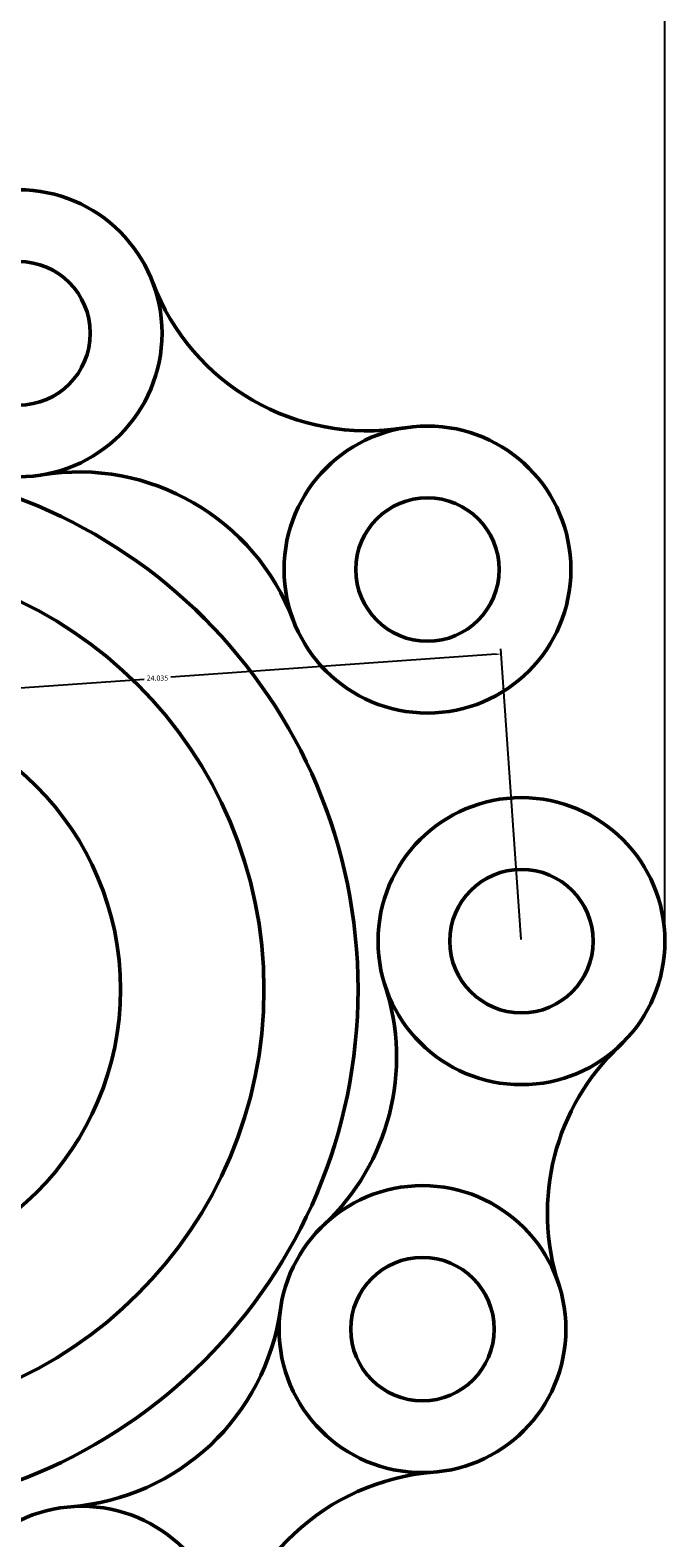
# Model space of a CAD drawing. Units: inches. Extents: x 413 to 622, y 326 to 447.
# Tile 14 of 15: x 600 to 622, y 367 to 420. Entities that reach past the tile are written whole.
import ezdxf

# ---------------------------------------------------------------- set-up
doc = ezdxf.new("R2010")
doc.units = ezdxf.units.IN
doc.header["$MEASUREMENT"] = 0
doc.layers.add('M-DIMS', color=2, linetype='Continuous', lineweight=18)
doc.layers.add('M-OUTL', color=7, linetype='Continuous', lineweight=50)
doc.styles.get("Standard").update_dxf_attribs({"font": 'arial.ttf'})
doc.dimstyles.get("Standard").update_dxf_attribs({"dimtxt": 0.18, "dimasz": 0.18, "dimexe": 0.18, "dimexo": 0.0625, "dimgap": 0.09, "dimtad": 0, "dimtih": 1, "dimtoh": 1, "dimdec": 4, "dimzin": 0, "dimdsep": 46, "dimtxsty": 'Standard', "dimcen": 0.09, "dimadec": 0, "dimazin": 0, "dimtfac": 1, "dimtdec": 4, "dimtofl": 0, "dimtmove": 0, "dimatfit": 3, "dimfxl": 1, "dimtolj": 1, "dimtzin": 0, "dimarcsym": 0})

# ---------------------------------------------------------------- blocks, each defined once
blk = doc.blocks.new('CHAIN-ROLLER-PIN')
for radius in [5, 2.5]:
    blk.add_circle((5, 5), radius)
blk = doc.blocks.new('SPROCKET-HUB-BORE')
for radius in [15, 10]:
    blk.add_circle((15, 15), radius)
blk = doc.blocks.new('*D11')
at = {"layer": 'Defpoints', "color": 0, "transparency": 16777216}
for p in [(621.66, 446.422), (621.66, 388.074), (423.314, 378.888)]:
    blk.add_point(p, dxfattribs=at)
at = {"layer": 'M-DIMS', "color": 0, "lineweight": -2, "transparency": 16777216}
for p, q in [((423.314, 378.95), (423.314, 446.602)), ((621.66, 388.137), (621.66, 446.602)), ((423.494, 446.422), (522.031, 446.422)), ((621.48, 446.422), (522.943, 446.422))]:
    blk.add_line(p, q, dxfattribs=at)
at = {"layer": 'M-DIMS', "color": 0, "transparency": 16777216}
for points in [[(423.494, 446.452), (423.494, 446.392), (423.314, 446.422)], [(621.48, 446.452), (621.48, 446.392), (621.66, 446.422)]]:
    blk.add_solid(points, dxfattribs=at)
at = {"layer": 'M-DIMS', "color": 0, "transparency": 16777216, "insert": (522.487, 446.422), "char_height": 0.18, "attachment_point": 5}
blk.add_mtext('\\A1;198.35', dxfattribs=at)
blk = doc.blocks.new('*D15')
at = {"layer": 'Defpoints', "color": 0, "transparency": 16777216}
for p in [(615.958, 398.08), (616.66, 388.074), (592.684, 386.392)]:
    blk.add_point(p, dxfattribs=at)
at = {"layer": 'M-DIMS', "color": 0, "lineweight": -2, "transparency": 16777216}
for p, q in [((616.656, 388.136), (615.945, 398.26)), ((615.778, 398.067), (604.435, 397.271)), ((592.161, 396.41), (603.504, 397.206)), ((592.679, 386.454), (591.969, 396.577))]:
    blk.add_line(p, q, dxfattribs=at)
at = {"layer": 'M-DIMS', "color": 0, "transparency": 16777216}
for points in [[(615.776, 398.097), (615.78, 398.037), (615.958, 398.08)], [(592.159, 396.44), (592.163, 396.38), (591.981, 396.397)]]:
    blk.add_solid(points, dxfattribs=at)
at = {"layer": 'M-DIMS', "color": 0, "transparency": 16777216, "insert": (603.97, 397.239), "char_height": 0.18, "attachment_point": 5}
blk.add_mtext('\\A1;24.035', dxfattribs=at)
blk = doc.blocks.new('*D25')
at = {"layer": 'Defpoints', "color": 0, "transparency": 16777216}
for p in [(574.404, 386.392), (610.964, 386.391)]:
    blk.add_point(p, dxfattribs=at)
at = {"layer": 'M-DIMS', "color": 0, "lineweight": -2, "transparency": 16777216}
for p, q in [((563.436, 386.392), (574.224, 386.392)), ((592.594, 386.392), (592.774, 386.392)), ((592.684, 386.302), (592.684, 386.482))]:
    blk.add_line(p, q, dxfattribs=at)
at = {"layer": 'M-DIMS', "color": 0, "transparency": 16777216}
blk.add_solid([(574.224, 386.422), (574.224, 386.362), (574.404, 386.392)], dxfattribs=at)
at = {"layer": 'M-DIMS', "color": 0, "transparency": 16777216, "insert": (562.944, 386.392), "char_height": 0.18, "attachment_point": 5}
blk.add_mtext('\\A1;∅36.56', dxfattribs=at)

msp = doc.modelspace()

# ---------------------------------------------------------------- linework, layer by layer
at = {"layer": 'M-OUTL'}
msp.add_circle((592.6836, 386.3915), 18.28, dxfattribs=at)
for centre, start, end in [((611.2884, 413.8505), 200.72313, 279.27687), ((601.2252, 396.4204), 20.72313, 99.27687), ((604.3052, 384.0295), 313.22911, 18.127), ((625.5639, 378.602), 133.22911, 198.127), ((600.3328, 376.3466), 274.43512, 352.08959), ((614.2144, 361.5964), 94.43512, 172.08959)]:
    msp.add_arc(centre, 8, start, end, dxfattribs=at)

# ---------------------------------------------------------------- block references
for name, p in [('CHAIN-ROLLER-PIN', (594.1299, 404.2509)), ('CHAIN-ROLLER-PIN', (608.3845, 396.021)), ('SPROCKET-HUB-BORE', (577.684, 371.392)), ('CHAIN-ROLLER-PIN', (611.6604, 383.0746)), ('CHAIN-ROLLER-PIN', (608.2095, 369.5579)), ('CHAIN-ROLLER-PIN', (596.3385, 358.386))]:
    msp.add_blockref(name, p, dxfattribs=at)

# ---------------------------------------------------------------- dimensions: what is measured, and where the dimension line sits
at = {"layer": 'M-DIMS'}
dim = msp.add_linear_dim(base=(621.66, 446.422), p1=(423.3136, 378.8878), p2=(621.66, 388.0741), dimstyle='Standard', override={"dimdec": 2, "dimlfac": 1, "dimrnd": 0, "dimzin": 0, "dimdsep": 46, "dimlunit": 2}, dxfattribs=at)
dim.commit()
dim.dimension.update_dxf_attribs({"geometry": '*D11', "text_midpoint": (522.4868, 446.422)})
dim = msp.add_linear_dim(base=(615.9578, 398.08), p1=(592.6836, 386.3915), p2=(616.66, 388.0741), angle=4.01433, dimstyle='Standard', override={"dimdec": 3, "dimlfac": 1, "dimrnd": 0, "dimzin": 0, "dimdsep": 46, "dimlunit": 2}, dxfattribs=at)
dim.commit()
dim.dimension.update_dxf_attribs({"geometry": '*D15', "text_midpoint": (603.9696, 397.2387)})
dim = msp.add_diameter_dim_2p(p1=(610.9636, 386.391), p2=(574.4036, 386.392), dimstyle='Standard', override={"dimdec": 2, "dimlfac": 1, "dimrnd": 0, "dimzin": 0, "dimdsep": 46, "dimlunit": 2}, dxfattribs=at)
dim.commit()
dim.dimension.update_dxf_attribs({"geometry": '*D25', "text_midpoint": (563.4356, 386.3923), "dimtype": 163})

doc.saveas('drawing.dxf')
